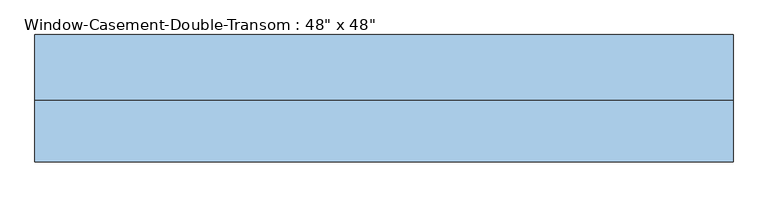
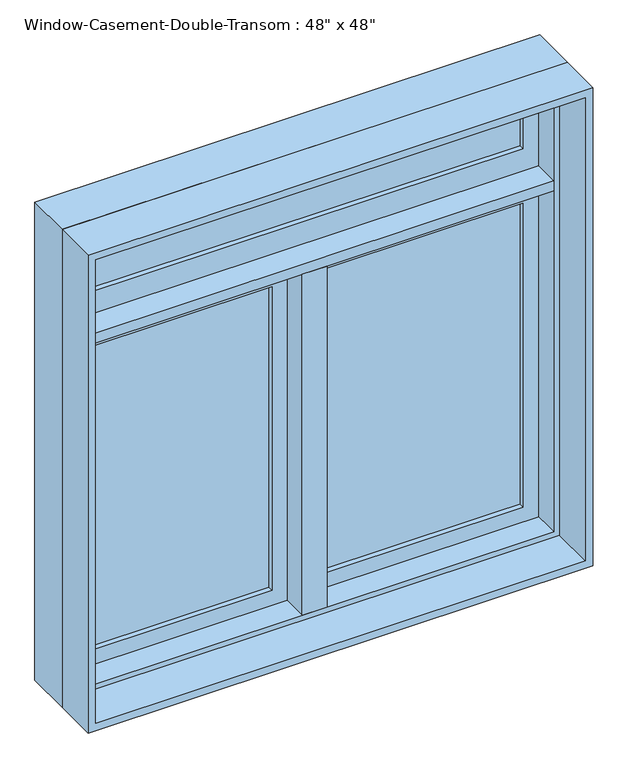
"""IFC4 building model written with IfcOpenShell, lengths in millimetres: window geometry."""

from ifc_helpers import new_model, si_unit, frame, origin, place, context, project, spatial, polyline, outline, extrude, faceted_brep, source, transform, mapped, element, save


def window_ba962a69(model_context):
    return source(origin(), model_context, "Body", "SolidModel", [
        faceted_brep([(577.85, 69.85, 2101.85), (577.85, 6.35, 2101.85), (-577.85, 6.35, 2101.85), (-577.85, 69.85, 2101.85), (596.9, 120.65, 2120.9), (596.9, 69.85, 2120.9), (-596.9, 69.85, 2120.9), (-596.9, 120.65, 2120.9), (609.6, 6.35, 2133.6), (609.6, 120.65, 2133.6), (-609.6, 120.65, 2133.6), (-609.6, 6.35, 2133.6), (-577.85, 6.35, 946.15), (-577.85, 69.85, 946.15), (-596.9, 69.85, 927.1), (-596.9, 120.65, 927.1), (-609.6, 120.65, 914.4), (-609.6, 6.35, 914.4), (577.85, 6.35, 946.15), (577.85, 69.85, 946.15), (596.9, 69.85, 927.1), (596.9, 120.65, 927.1), (609.6, 120.65, 914.4), (609.6, 6.35, 914.4)], [[[0, 1, 2, 3]], [[4, 5, 6, 7]], [[8, 9, 10, 11]], [[3, 2, 12, 13]], [[7, 6, 14, 15]], [[11, 10, 16, 17]], [[13, 12, 18, 19]], [[15, 14, 20, 21]], [[17, 16, 22, 23]], [[11, 17, 23, 8], [1, 18, 12, 2]], [[19, 18, 1, 0]], [[5, 20, 14, 6], [3, 13, 19, 0]], [[21, 20, 5, 4]], [[23, 22, 9, 8]], [[9, 22, 16, 10], [7, 15, 21, 4]]]),
        extrude(outline(polyline([(2133.6, -609.6), (914.4, -609.6), (914.4, 609.6), (2133.6, 609.6), (2133.6, -609.6)]), holes=[polyline([(2114.55, 590.55), (933.45, 590.55), (933.45, -590.55), (2114.55, -590.55), (2114.55, 590.55)])]), frame((0.0, -101.6, 0.0), z_axis=(0.0, 1.0, 0.0), x_axis=(0.0, 0.0, 1.0)), (0.0, 0.0, 1.0), 107.95),
        extrude(outline(polyline([(927.1, 596.9), (1816.1, 596.9), (1816.1, 9.525), (927.1, 9.525), (927.1, 596.9)]), holes=[polyline([(984.25, 66.675), (1758.95, 66.675), (1758.95, 539.75), (984.25, 539.75), (984.25, 66.675)])]), frame((0.0, 69.85, 0.0), z_axis=(0.0, 1.0, 0.0), x_axis=(0.0, 0.0, 1.0)), (0.0, 0.0, 1.0), 44.45),
        extrude(outline(polyline([(1816.1, -596.9), (927.1, -596.9), (927.1, -9.525), (1816.1, -9.525), (1816.1, -596.9)]), holes=[polyline([(1758.95, -66.675), (984.25, -66.675), (984.25, -539.75), (1758.95, -539.75), (1758.95, -66.675)])]), frame((0.0, 69.85, 0.0), z_axis=(0.0, 1.0, 0.0), x_axis=(0.0, 0.0, 1.0)), (0.0, 0.0, 1.0), 44.45),
        extrude(outline(polyline([(539.75, 101.6), (539.75, 95.25), (66.675, 95.25), (66.675, 101.6), (539.75, 101.6)])), frame((0.0, 0.0, 984.25), z_axis=(0.0, 0.0, 1.0), x_axis=(1.0, 0.0, 0.0)), (0.0, 0.0, 1.0), 774.7),
        extrude(outline(polyline([(66.675, 82.55), (66.675, 88.9), (539.75, 88.9), (539.75, 82.55), (66.675, 82.55)])), frame((0.0, 0.0, 984.25), z_axis=(0.0, 0.0, 1.0), x_axis=(1.0, 0.0, 0.0)), (0.0, 0.0, 1.0), 774.7),
        extrude(outline(polyline([(-66.675, 101.6), (-66.675, 95.25), (-539.75, 95.25), (-539.75, 101.6), (-66.675, 101.6)])), frame((0.0, 0.0, 984.25), z_axis=(0.0, 0.0, 1.0), x_axis=(1.0, 0.0, 0.0)), (0.0, 0.0, 1.0), 774.7),
        extrude(outline(polyline([(-539.75, 82.55), (-539.75, 88.9), (-66.675, 88.9), (-66.675, 82.55), (-539.75, 82.55)])), frame((0.0, 0.0, 984.25), z_axis=(0.0, 0.0, 1.0), x_axis=(1.0, 0.0, 0.0)), (0.0, 0.0, 1.0), 774.7),
        faceted_brep([(9.525, 120.65, 1816.1), (-9.525, 120.65, 1816.1), (-9.525, 69.85, 1816.1), (-30.1625, 69.85, 1816.1), (-30.1625, 6.35, 1816.1), (30.1625, 6.35, 1816.1), (30.1625, 69.85, 1816.1), (9.525, 69.85, 1816.1), (9.525, 120.65, 927.1), (9.525, 69.85, 927.1), (-9.525, 69.85, 927.1), (-9.525, 120.65, 927.1), (-9.525, 69.85, 946.15), (-30.1625, 69.85, 946.15), (-30.1625, 6.35, 946.15), (30.1625, 6.35, 946.15), (30.1625, 69.85, 946.15), (9.525, 69.85, 946.15)], [[[0, 1, 2, 3, 4, 5, 6, 7]], [[8, 9, 10, 11]], [[1, 0, 8, 11]], [[2, 1, 11, 10, 12]], [[3, 2, 12, 13]], [[4, 3, 13, 14]], [[5, 4, 14, 15]], [[6, 5, 15, 16]], [[7, 6, 16, 17]], [[0, 7, 17, 9, 8]], [[17, 12, 10, 9]], [[12, 17, 16, 15, 14, 13]]]),
        extrude(outline(polyline([(539.75, 101.6), (539.75, 95.25), (-539.75, 95.25), (-539.75, 101.6), (539.75, 101.6)])), frame((0.0, 0.0, 1898.65), z_axis=(0.0, 0.0, 1.0), x_axis=(1.0, 0.0, 0.0)), (0.0, 0.0, 1.0), 165.1),
        extrude(outline(polyline([(-539.75, 82.55), (-539.75, 88.9), (539.75, 88.9), (539.75, 82.55), (-539.75, 82.55)])), frame((0.0, 0.0, 1898.65), z_axis=(0.0, 0.0, 1.0), x_axis=(1.0, 0.0, 0.0)), (0.0, 0.0, 1.0), 165.1),
        extrude(outline(polyline([(596.9, 120.65), (596.9, 69.85), (577.85, 69.85), (577.85, 6.35), (-577.85, 6.35), (-577.85, 69.85), (-596.9, 69.85), (-596.9, 120.65), (596.9, 120.65)])), frame((0.0, 0.0, 1816.1), z_axis=(0.0, 0.0, 1.0), x_axis=(1.0, 0.0, 0.0)), (0.0, 0.0, 1.0), 25.4),
        extrude(outline(polyline([(2120.9, -596.9), (1841.5, -596.9), (1841.5, 596.9), (2120.9, 596.9), (2120.9, -596.9)]), holes=[polyline([(2063.75, 539.75), (1898.65, 539.75), (1898.65, -539.75), (2063.75, -539.75), (2063.75, 539.75)])]), frame((0.0, 69.85, 0.0), z_axis=(0.0, 1.0, 0.0), x_axis=(0.0, 0.0, 1.0)), (0.0, 0.0, 1.0), 44.45),
    ])


if __name__ == "__main__":
    model = new_model("IFC4")
    model_context = context("Model", 3, world=origin())
    ifc_project = project(units=[si_unit("LENGTHUNIT", "METRE", prefix="MILLI")], contexts=[model_context])
    site = spatial("IfcSite", under=ifc_project)
    building = spatial("IfcBuilding", under=site)
    placement = place(None, origin())
    window_shape = window_ba962a69(model_context)
    element("IfcWindow", 1, ObjectType="Window-Casement-Double-Transom : 48\" x 48\"", at=placement, inside=building, context=model_context, shape_type="MappedRepresentation", body=[
        mapped(window_shape, transform((0.0, 0.0, 0.0), x_axis=(1.0, 0.0, 0.0), y_axis=(0.0, 1.0, 0.0), z_axis=(0.0, 0.0, 1.0))),
    ])
    save(model, "model.ifc")

# Revit data of these elements
# Type "Window-Casement-Double-Transom : 48\" x 48\""
#   Type Mark = "18"
#   Fire Rating = "0.5h"
#   Assembly Code = "B2020100"
#   Analytic Construction = "Double glazing - domestic"
#   Window Inset [instance default] = 0' - 0"
#   Wall Thickness [instance default] = 0' - 6"
#   Interior Wall Closure [instance default] = 0' - 2 1/4"
#   Half Width = 2' - 0"
#   Visual Light Transmittance = 0.81
#   Transom Height = 1' - 0"
#   Thermal Resistance (R) = 1.8146 (h·ft²·°F)/BTU
#   Solar Heat Gain Coefficient = 0.76
#   Rough Width = 4' - 0 1/2"
#   Rough Height = 4' - 0 1/2"
#   Open Window Height = 3' - 0"
#   Height = 4' - 0"
#   Heat Transfer Coefficient (U) = 0.5511 BTU/(h·ft²·°F)
#   Frame Extension [instance default] = 0' - 0 1/4"
#   Exterior Wall Closure [instance default] = 0' - 1 1/4"
#   Extension Jamb [instance default] = 0' - 2 1/4"
#   Default Sill Height = 3' - 0"
#   Width = 4' - 0"
#   Muntin Visibility = yes
#   Interior Trim Visibility [instance default] = yes
#   Exterior Trim Visibility [instance default] = yes
#   Extension Jamb Visibility [instance default] = yes
#   Interior Trim Material = Wood - Stained
#   Muntin Pattern = Muntin Pattern_2x2 : Muntin Pattern_2x2
#   Interior Trim = Trim-Window-Interior-Flat : Picture Frame
#   Interior Frame Material = Wood - Stained
#   Glass Panel Material = Glass
#   Exterior Trim Material = Clad - White
#   Exterior Trim = Trim-Window-Exterior-Flat : with Sill
#   Exterior Frame Material = Clad - White
#   Wall Closure = (empty or 0)
# Element 1 (IfcWindow, "Window-Casement-Double-Transom : 48\" x 48\"")
#   Wall Thickness = 0' - 8"
#   Extension Jamb = 0' - 4 1/4"
#   Materials on its faces: "Wood - Stained", "Glass", "Clad - White"
# Materials
#   "Wood - Stained": class "Wood", colour RGB 224 178 126, transparency 0, Cost = 0
#   "Glass": class "Glass", colour RGB 0 128 192, transparency 0.75, Description = "Soda Lime Glass", Cost = 0
#   "Clad - White": class "Wood", colour RGB 242 242 238, transparency 0, Cost = 0
